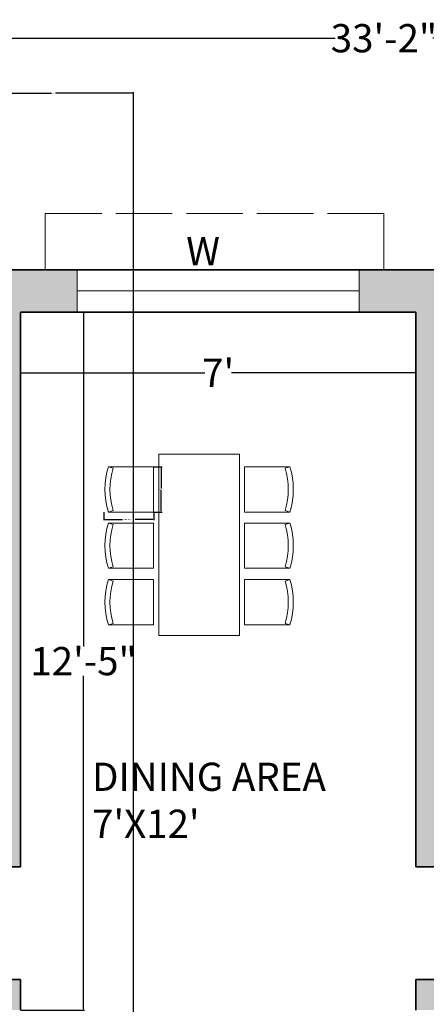
# Model space of a CAD drawing. Units: inches. Extents: x -5 to 482, y -460 to 66.
# Tile 30 of 31: x 154 to 241, y -143 to 66. Entities that reach past the tile are written whole.
import ezdxf

# ---------------------------------------------------------------- set-up
doc = ezdxf.new("R2010")
doc.units = ezdxf.units.IN
doc.header["$MEASUREMENT"] = 0
doc.linetypes.add('ACAD_ISO02W100', pattern=[15, 12, -3])
for name, color, linetype, lineweight in [('A-ANNO-DIMS', 2, 'Continuous', 18), ('A-ANNO-TEXT', 7, 'Continuous', 18), ('A-AREA-IDEN', 7, 'Continuous', 18), ('A-FURN', 8, 'Continuous', 18), ('A-GLAZ', 4, 'Continuous', 18), ('A-GLAZ-OVHD', 4, 'ACAD_ISO02W100', 13), ('A-WALL', 7, 'Continuous', 35), ('A-WALL-PATT', 152, 'Continuous', 13)]:
    doc.layers.add(name, color=color, linetype=linetype, lineweight=lineweight)
doc.styles.get("Standard").update_dxf_attribs({"font": 'arial.ttf'})
doc.dimstyles.get("Standard").update_dxf_attribs({"dimtxt": 0.18, "dimasz": 0.18, "dimexe": 0.18, "dimexo": 0.0625, "dimgap": 0.09, "dimtad": 0, "dimtih": 1, "dimtoh": 1, "dimdec": 0, "dimzin": 0, "dimdsep": 46, "dimlunit": 3, "dimtxsty": 'Standard', "dimcen": 0.09, "dimadec": 0, "dimazin": 0, "dimtfac": 1, "dimtdec": 0, "dimtofl": 0, "dimtmove": 0, "dimatfit": 3, "dimfxl": 1, "dimtolj": 1, "dimtzin": 0, "dimarcsym": 0})

# ---------------------------------------------------------------- blocks, each defined once
blk = doc.blocks.new('*D3')
at = {"layer": 'A-ANNO-DIMS', "color": 0, "lineweight": -2, "transparency": 16777216}
for p, q in [((32.88, 13.21), (32.88, 62.61)), ((33.06, 62.43), (221.23, 62.43)), ((430.2, 62.43), (242.02, 62.43)), ((430.38, 13.21), (430.38, 62.61))]:
    blk.add_line(p, q, dxfattribs=at)
at = {"layer": 'A-ANNO-DIMS', "color": 0, "transparency": 16777216}
for points in [[(33.06, 62.46), (33.06, 62.4), (32.88, 62.43)], [(430.2, 62.46), (430.2, 62.4), (430.38, 62.43)]]:
    blk.add_solid(points, dxfattribs=at)
at = {"layer": 'Defpoints', "color": 0, "transparency": 16777216}
for p in [(430.38, 62.43), (32.88, 13.15), (430.38, 13.15)]:
    blk.add_point(p, dxfattribs=at)
at = {"layer": 'A-ANNO-DIMS', "color": 0, "transparency": 16777216, "insert": (231.63, 62.43), "char_height": 6, "attachment_point": 5}
blk.add_mtext('\\A1;33\'-2"', dxfattribs=at)
blk = doc.blocks.new('*D7')
at = {"layer": 'A-ANNO-DIMS', "color": 0, "lineweight": -2, "transparency": 16777216}
for p, q in [((154.38, -11.36), (154.38, -8.57)), ((154.56, -8.75), (193.55, -8.75)), ((238.2, -8.75), (199.2, -8.75)), ((238.38, -11.36), (238.38, -8.57))]:
    blk.add_line(p, q, dxfattribs=at)
at = {"layer": 'A-ANNO-DIMS', "color": 0, "transparency": 16777216}
for points in [[(154.56, -8.72), (154.56, -8.78), (154.38, -8.75)], [(238.2, -8.72), (238.2, -8.78), (238.38, -8.75)]]:
    blk.add_solid(points, dxfattribs=at)
at = {"layer": 'Defpoints', "color": 0, "transparency": 16777216}
for p in [(238.38, -8.75), (154.38, -11.42), (238.38, -11.42)]:
    blk.add_point(p, dxfattribs=at)
at = {"layer": 'A-ANNO-DIMS', "color": 0, "transparency": 16777216, "insert": (196.38, -8.75), "char_height": 6, "attachment_point": 5}
blk.add_mtext("\\A1;7'", dxfattribs=at)
blk = doc.blocks.new('*D8')
at = {"layer": 'A-ANNO-DIMS', "color": 0, "lineweight": -2, "transparency": 16777216}
for p, q in [((154.44, 4.15), (167.95, 4.15)), ((167.77, 3.97), (167.77, -66.95)), ((167.77, -144.17), (167.77, -73.25)), ((154.44, -144.35), (167.95, -144.35))]:
    blk.add_line(p, q, dxfattribs=at)
at = {"layer": 'A-ANNO-DIMS', "color": 0, "transparency": 16777216}
for points in [[(167.74, 3.97), (167.8, 3.97), (167.77, 4.15)], [(167.74, -144.17), (167.8, -144.17), (167.77, -144.35)]]:
    blk.add_solid(points, dxfattribs=at)
at = {"layer": 'Defpoints', "color": 0, "transparency": 16777216}
for p in [(154.38, 4.15), (167.77, 4.15), (154.38, -144.35)]:
    blk.add_point(p, dxfattribs=at)
at = {"layer": 'A-ANNO-DIMS', "color": 0, "transparency": 16777216, "insert": (167.77, -70.1), "char_height": 6, "attachment_point": 5}
blk.add_mtext('\\A1;12\'-5"', dxfattribs=at)
blk = doc.blocks.new('WIN-GLAZ-60IN')
for p, q in [((0, 9), (60, 9)), ((0, 4.5), (60, 4.5)), ((60, 0), (0, 0))]:
    blk.add_line(p, q)
blk = doc.blocks.new('WIN-SHADE-72IN')
for p, q in [((0, 12), (72, 12)), ((0, 12), (0, 0)), ((72, 12), (72, 0))]:
    blk.add_line(p, q)
blk = doc.blocks.new('DINING-CHAIR')
for p, q in [((0.75, 9.63), (1.77, 9.31)), ((0.75, 0), (1.77, 0.32))]:
    blk.add_line(p, q)
blk.add_lwpolyline([(0.74, 9.63), (10.37, 9.63), (10.37, 0), (0.74, 0, -0.153703), (0.74, 9.63)], format="xyb")
for radius in [15.89, 14.82]:
    blk.add_arc((15.89, 4.82), radius, 162.3544, 197.6456)
blk = doc.blocks.new('*D47')
at = {"layer": 'A-ANNO-DIMS', "color": 0, "lineweight": -2, "transparency": 16777216}
for p, q in [((172.05, -38.43), (172.05, -40.14)), ((182.68, -38.43), (182.68, -40.14)), ((172.23, -39.96), (176.02, -39.96)), ((182.5, -39.96), (178.71, -39.96))]:
    blk.add_line(p, q, dxfattribs=at)
at = {"layer": 'A-ANNO-DIMS', "color": 0, "transparency": 16777216}
for points in [[(172.23, -39.93), (172.23, -39.99), (172.05, -39.96)], [(182.5, -39.93), (182.5, -39.99), (182.68, -39.96)]]:
    blk.add_solid(points, dxfattribs=at)
at = {"layer": 'Defpoints', "color": 0, "transparency": 16777216}
for p in [(172.05, -38.37), (182.68, -38.37), (182.68, -39.96)]:
    blk.add_point(p, dxfattribs=at)
at = {"layer": 'A-ANNO-DIMS', "color": 0, "transparency": 16777216, "insert": (177.37, -39.96), "char_height": 0.18, "attachment_point": 5}
blk.add_mtext('\\A1;CHAIR 0\'-10 1/2" TYP.', dxfattribs=at)
blk = doc.blocks.new('*D48')
at = {"layer": 'A-ANNO-DIMS', "color": 0, "lineweight": -2, "transparency": 16777216}
for p, q in [((182.74, -28.73), (184.45, -28.73)), ((184.27, -28.91), (184.27, -33.37)), ((184.27, -38.19), (184.27, -33.73)), ((182.74, -38.37), (184.45, -38.37))]:
    blk.add_line(p, q, dxfattribs=at)
at = {"layer": 'A-ANNO-DIMS', "color": 0, "transparency": 16777216}
for points in [[(184.24, -28.91), (184.3, -28.91), (184.27, -28.73)], [(184.24, -38.19), (184.3, -38.19), (184.27, -38.37)]]:
    blk.add_solid(points, dxfattribs=at)
at = {"layer": 'Defpoints', "color": 0, "transparency": 16777216}
for p in [(182.68, -28.73), (184.27, -28.73), (182.68, -38.37)]:
    blk.add_point(p, dxfattribs=at)
at = {"layer": 'A-ANNO-DIMS', "color": 0, "transparency": 16777216, "insert": (184.27, -33.55), "char_height": 0.18, "attachment_point": 5}
blk.add_mtext('\\A1;0\'-9 1/2" TYP.', dxfattribs=at)
blk = doc.blocks.new('*D73')
at = {"layer": 'A-ANNO-DIMS', "color": 0, "lineweight": -2, "transparency": 16777216}
for p, q in [((144.38, -295.8), (144.38, 50.93)), ((144.56, 50.75), (160.98, 50.75)), ((178.2, 50.75), (161.78, 50.75)), ((178.38, -295.8), (178.38, 50.93))]:
    blk.add_line(p, q, dxfattribs=at)
at = {"layer": 'A-ANNO-DIMS', "color": 0, "transparency": 16777216}
for points in [[(144.56, 50.78), (144.56, 50.72), (144.38, 50.75)], [(178.2, 50.78), (178.2, 50.72), (178.38, 50.75)]]:
    blk.add_solid(points, dxfattribs=at)
at = {"layer": 'Defpoints', "color": 0, "transparency": 16777216}
for p in [(178.38, 50.75), (144.38, -295.86), (178.38, -295.86)]:
    blk.add_point(p, dxfattribs=at)
at = {"layer": 'A-ANNO-DIMS', "color": 0, "transparency": 16777216, "insert": (161.38, 50.75), "char_height": 0.18, "attachment_point": 5}
blk.add_mtext('\\A1;2\'-10"', dxfattribs=at)

msp = doc.modelspace()

# ---------------------------------------------------------------- hatches: boundary and pattern name
at = {"layer": 'A-WALL-PATT'}
h = msp.add_hatch(color=256, dxfattribs=at)
h.dxf.hatch_style = 1
h.paths.add_polyline_path([(149.38, -412.85), (144.38, -412.85), (144.38, -283.85), (144.38, -279.35), (133.88, -279.35), (133.88, -283.85), (139.88, -283.85), (139.88, -412.85), (133.51, -412.85), (133.51, -413.92), (102.65, -413.92), (102.65, -421.02), (133.51, -421.02), (133.51, -421.85), (149.38, -421.85)])
h.paths.add_polyline_path([(226.05, -412.85), (218.88, -412.85), (218.88, -350.85), (262.88, -350.85), (262.88, -386.85), (267.38, -386.85), (267.38, -283.85), (270.38, -283.85), (270.38, -279.35), (244.88, -279.35), (244.88, -283.85), (262.88, -283.85), (262.88, -346.35), (218.88, -346.35), (218.88, -283.85), (220.88, -283.85), (220.88, -279.35), (214.38, -279.35), (214.38, -283.85), (214.38, -412.85), (209.38, -412.85), (209.38, -421.85), (226.05, -421.85)])
h.paths.add_polyline_path([(315.81, -412.85), (250.05, -412.85), (250.05, -421.85), (315.81, -421.85)])
h.paths.add_polyline_path([(430.38, -378.35), (421.38, -378.35), (421.38, -412.85), (375.81, -412.85), (375.81, -421.85), (430.38, -421.85)])
h.paths.add_polyline_path([(78.69, -413.92), (47.68, -413.92), (47.68, -412.85), (41.88, -412.85), (41.88, -283.85), (109.88, -283.85), (109.88, -279.35), (41.88, -279.35), (41.88, -241.85), (32.88, -241.85), (32.88, -421.85), (47.68, -421.85), (47.68, -421.02), (78.69, -421.02)])
h.paths.add_polyline_path([(41.88, -144.35), (154.38, -144.35), (154.38, -137.85), (149.88, -137.85), (149.88, -139.85), (41.88, -139.85), (41.88, -97.85), (32.88, -97.85), (32.88, -181.85), (41.88, -181.85)])
h.paths.add_polyline_path([(430.38, -241.85), (421.38, -241.85), (421.38, -279.35), (309.38, -279.35), (309.38, -170.35), (304.88, -170.35), (304.88, -279.35), (294.38, -279.35), (294.38, -283.85), (421.38, -283.85), (421.38, -318.35), (430.38, -318.35)])
h.paths.add_polyline_path([(430.38, -119.85), (421.38, -119.85), (421.38, -139.85), (419.38, -139.85), (419.38, -144.35), (421.38, -144.35), (421.38, -181.85), (430.38, -181.85)])
h.paths.add_polyline_path([(395.38, -139.85), (377.38, -139.85), (377.38, -75.85), (421.38, -75.85), (421.38, -95.85), (430.38, -95.85), (430.38, -45.6), (421.38, -45.6), (421.38, -71.35), (377.38, -71.35), (377.38, -22.85), (372.88, -22.85), (372.88, -139.85), (242.88, -139.85), (242.88, -137.85), (238.38, -137.85), (238.38, -144.35), (304.88, -144.35), (304.88, -146.35), (309.38, -146.35), (309.38, -144.35), (395.38, -144.35)])
h.paths.add_polyline_path([(65.88, 13.15), (32.88, 13.15), (32.88, -37.85), (41.88, -37.85), (41.88, 4.15), (65.88, 4.15)])
h.paths.add_polyline_path([(166.38, 13.15), (125.88, 13.15), (125.88, 4.15), (149.88, 4.15), (149.88, -113.85), (154.38, -113.85), (154.38, 4.15), (166.38, 4.15)])
h.paths.add_polyline_path([(277.88, 13.15), (226.38, 13.15), (226.38, 4.15), (238.38, 4.15), (238.38, -113.85), (242.88, -113.85), (242.88, 4.15), (277.88, 4.15)])
h.paths.add_polyline_path([(430.38, 13.15), (337.88, 13.15), (337.88, 4.15), (372.88, 4.15), (372.88, 1.15), (377.38, 1.15), (377.38, 4.15), (421.38, 4.15), (421.38, -21.6), (430.38, -21.6)])

# ---------------------------------------------------------------- linework, layer by layer
at = {"layer": 'A-FURN'}
msp.add_lwpolyline([(200.89, -64.61), (183.77, -64.61), (183.77, -26.07), (200.89, -26.07)], close=True, dxfattribs=at)
at = {"layer": 'A-GLAZ'}
for p, q in [((166.38, 4.15), (166.38, 13.15)), ((226.38, 13.15), (226.38, 4.15))]:
    msp.add_line(p, q, dxfattribs=at)
at = {"layer": 'A-WALL'}
for p, q in [((32.88, 13.15), (430.38, 13.15)), ((154.38, 4.15), (154.38, -113.85)), ((154.38, 4.15), (238.38, 4.15)), ((238.38, 4.15), (238.38, -113.85)), ((149.88, -113.85), (154.38, -113.85)), ((242.88, -113.85), (238.38, -113.85)), ((149.88, -137.85), (154.38, -137.85)), ((154.38, -137.85), (154.38, -144.35)), ((242.88, -137.85), (238.38, -137.85)), ((238.38, -137.85), (238.38, -144.35))]:
    msp.add_line(p, q, dxfattribs=at)

# ---------------------------------------------------------------- block references
at = {"layer": 'A-FURN'}
for p in [(172.3, -38.37), (172.3, -50.34), (172.3, -62.38)]:
    msp.add_blockref('DINING-CHAIR', p, dxfattribs=at)
at = {"layer": 'A-FURN', "extrusion": (0, 0, -1), "zscale": -1}
for p in [(-212.36, -38.37), (-212.36, -50.34), (-212.36, -62.38)]:
    msp.add_blockref('DINING-CHAIR', p, dxfattribs=at)
at = {"layer": 'A-GLAZ'}
msp.add_blockref('WIN-GLAZ-60IN', (166.38, 4.15), dxfattribs=at)
at = {"layer": 'A-GLAZ-OVHD'}
msp.add_blockref('WIN-SHADE-72IN', (159.63, 13.15), dxfattribs=at)

# ---------------------------------------------------------------- texts
at = {"layer": 'A-ANNO-TEXT', "insert": (189.58, 20.13), "char_height": 6, "attachment_point": 1}
msp.add_mtext('W', dxfattribs=at)
at = {"layer": 'A-AREA-IDEN', "insert": (169.57, -91.7), "char_height": 6, "width": 115.0787, "attachment_point": 1}
msp.add_mtext("DINING AREA\\P7'X12'", dxfattribs=at)

# ---------------------------------------------------------------- dimensions: what is measured, and where the dimension line sits
at = {"layer": 'A-ANNO-DIMS'}
for base, p1, p2, override, picture, middle in [((430.37673599, 62.43157193), (32.87673599, 13.15133597), (430.37673599, 13.15133597), {"dimtxt": 6, "dimclrd": 0, "dimclre": 0, "dimclrt": 0}, '*D3', (231.62673599, 62.43157193)), ((178.38, 50.75), (144.38, -295.86), (178.38, -295.86), {"dimdec": 1, "dimlfac": 1, "dimrnd": 0, "dimzin": 1, "dimdsep": 46, "dimlunit": 4, "dimfrac": 2}, '*D73', (161.38, 50.75)), ((238.38, -8.75), (154.38, -11.42), (238.38, -11.42), {"dimtxt": 6, "dimclrd": 0, "dimclre": 0, "dimclrt": 0}, '*D7', (196.38, -8.75))]:
    dim = msp.add_linear_dim(base=base, p1=p1, p2=p2, dimstyle='Standard', override=override, dxfattribs=at)
    dim.commit()
    dim.dimension.update_dxf_attribs({"geometry": picture, "text_midpoint": middle})
dim = msp.add_linear_dim(base=(167.76833102, 4.15133597), p1=(154.37673599, -144.34866403), p2=(154.37673599, 4.15133597), angle=90, dimstyle='Standard', override={"dimtxt": 6, "dimclrd": 0, "dimclre": 0, "dimclrt": 0}, dxfattribs=at)
dim.commit()
dim.dimension.update_dxf_attribs({"geometry": '*D8', "text_midpoint": (167.76833102, -70.09866403)})
dim = msp.add_linear_dim(base=(184.27, -28.73), p1=(182.68, -38.37), p2=(182.68, -28.73), angle=90, text='<> TYP.', dimstyle='Standard', override={"dimdec": 1, "dimlfac": 1, "dimrnd": 0, "dimzin": 1, "dimdsep": 46, "dimlunit": 4, "dimfrac": 2}, dxfattribs=at)
dim.commit()
dim.dimension.update_dxf_attribs({"geometry": '*D48', "text_midpoint": (184.27, -33.55)})
dim = msp.add_linear_dim(base=(182.68, -39.96), p1=(172.05, -38.37), p2=(182.68, -38.37), text='CHAIR <> TYP.', dimstyle='Standard', override={"dimdec": 1, "dimlfac": 1, "dimrnd": 0, "dimzin": 1, "dimdsep": 46, "dimlunit": 4, "dimfrac": 2}, dxfattribs=at)
dim.commit()
dim.dimension.update_dxf_attribs({"geometry": '*D47', "text_midpoint": (177.37, -39.96)})

doc.saveas('drawing.dxf')
